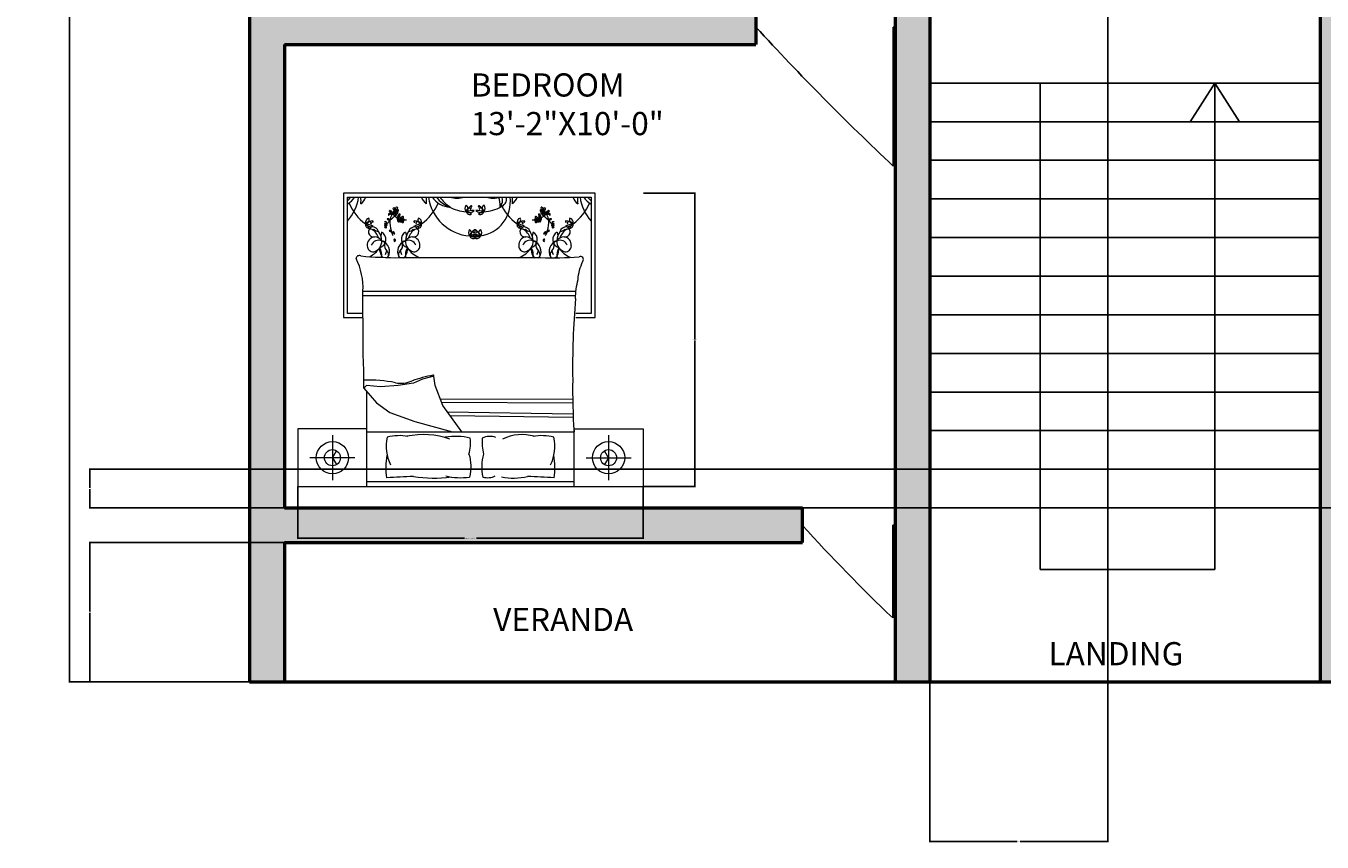
# Model space of a CAD drawing. Units: inches. Extents: x -17 to 536, y -817 to 53.
# Tile 1 of 9: x -17 to 319, y -817 to -606. Entities that reach past the tile are written whole.
import ezdxf

# ---------------------------------------------------------------- set-up
doc = ezdxf.new("R2010")
doc.units = ezdxf.units.IN
doc.header["$MEASUREMENT"] = 0
for name, color, linetype, lineweight in [('A-ANNO-DIMS', 2, 'Continuous', 18), ('A-AREA-IDEN', 7, 'Continuous', 18), ('A-DOOR', 4, 'Continuous', 25), ('A-FLOR-STRS', 7, 'Continuous', 25), ('A-FURN', 8, 'Continuous', 13), ('A-WALL', 7, 'Continuous', 50), ('A-WALL-PATT', 22, 'Continuous', 13)]:
    doc.layers.add(name, color=color, linetype=linetype, lineweight=lineweight)
doc.styles.get("Standard").update_dxf_attribs({"font": 'arial.ttf'})
doc.dimstyles.get("Standard").update_dxf_attribs({"dimtxt": 0.18, "dimasz": 0.18, "dimexe": 0.18, "dimexo": 0.0625, "dimgap": 0.09, "dimtad": 0, "dimtih": 1, "dimtoh": 1, "dimdec": 0, "dimzin": 0, "dimdsep": 46, "dimlunit": 3, "dimtxsty": 'Standard', "dimcen": 0.09, "dimadec": 0, "dimazin": 0, "dimtfac": 1, "dimtdec": 0, "dimtofl": 0, "dimtmove": 0, "dimatfit": 3, "dimfxl": 1, "dimtolj": 1, "dimtzin": 0, "dimarcsym": 0})

# ---------------------------------------------------------------- blocks, each defined once
blk = doc.blocks.new('*D2')
at = {"layer": 'A-ANNO-DIMS', "color": 0, "lineweight": -2, "transparency": 16777216}
for p, q in [((41.3, 11.55), (-5.38, 11.55)), ((-5.2, 11.37), (-5.2, -378.8)), ((-5.2, -775.27), (-5.2, -385.1)), ((41.3, -775.45), (-5.38, -775.45))]:
    blk.add_line(p, q, dxfattribs=at)
at = {"layer": 'A-ANNO-DIMS', "color": 0, "transparency": 16777216}
for points in [[(-5.23, 11.37), (-5.17, 11.37), (-5.2, 11.55)], [(-5.23, -775.27), (-5.17, -775.27), (-5.2, -775.45)]]:
    blk.add_solid(points, dxfattribs=at)
at = {"layer": 'Defpoints', "color": 0, "transparency": 16777216}
for p in [(41.37, 11.55), (-5.2, -775.45), (41.37, -775.45)]:
    blk.add_point(p, dxfattribs=at)
at = {"layer": 'A-ANNO-DIMS', "color": 0, "transparency": 16777216, "insert": (-5.2, -381.95), "char_height": 6, "attachment_point": 5}
blk.add_mtext('\\A1;65\'-7"', dxfattribs=at)
blk = doc.blocks.new('BED-WITH-NIGHTSTANDS-STANDARD')
for p, q in [((11.79, 75.95), (11.79, 43.78)), ((76.89, 75.95), (11.79, 75.95)), ((12.82, 74.91), (75.86, 74.91)), ((12.82, 44.81), (12.82, 74.91)), ((75.86, 74.91), (75.86, 44.81)), ((76.89, 43.78), (76.89, 75.95)), ((21.62, 65.86), (21.42, 64.85)), ((27.86, 65.86), (28.06, 64.85)), ((60.82, 65.86), (60.62, 64.85)), ((67.06, 65.86), (67.25, 64.85)), ((62.78, 59.23), (26.52, 59.23)), ((71.93, 50.46), (16.83, 50.46)), ((71.85, 49.35), (16.83, 49.35)), ((11.79, 43.78), (16.84, 43.78)), ((16.84, 44.81), (12.82, 44.81)), ((75.86, 44.81), (71.92, 44.81)), ((71.94, 43.78), (76.89, 43.78)), ((32.25, 27.79), (29.9, 26.71)), ((35.15, 28.52), (32.25, 27.79)), ((35.51, 26.17), (35.15, 28.52)), ((17.78, 26.17), (17.06, 25.44)), ((17.06, 25.44), (20.32, 21.65)), ((21.4, 25.8), (17.78, 26.17)), ((17.86, 0), (17.86, 24.51)), ((25.92, 26.17), (21.4, 25.8)), ((29.9, 26.71), (25.92, 26.17)), ((37.5, 20.92), (35.51, 26.17)), ((20.32, 21.65), (23.75, 19.12)), ((71.13, 22.47), (36.86, 22.61)), ((71.12, 21.55), (37.21, 21.69)), ((42.39, 14.11), (37.5, 20.92)), ((23.75, 19.12), (30.26, 16.77)), ((71.17, 18.74), (38.74, 19.2)), ((71.2, 17.82), (39.41, 18.27)), ((17.86, 14.11), (71.44, 14.11)), ((30.26, 16.77), (40, 14.11)), ((8.93, 13.28), (8.93, 1.61)), ((80.37, 13.28), (80.37, 1.61)), ((14.76, 7.44), (3.1, 7.44)), ((74.54, 7.44), (86.21, 7.44)), ((0, 0), (89.3, 0)), ((71.44, 1.15), (17.86, 1.15))]:
    blk.add_line(p, q)
for points in [[(16.87, 33.62, -0.001242), (16.83, 50.56, 0.127202), (15.04, 59.01)], [(71.82, 48.64, -0.056112), (72.47, 53.56, -0.095341), (73.73, 58.29)], [(22.99, 2.23, -0.074897), (23.1, 8.06, 0.472817)], [(44.23, 8.39, -0.14099), (44.41, 2.43, -0.235245)], [(48.05, 8.39, 0.14099), (47.87, 2.43, 0.235245)], [(66.31, 2.23, 0.074897), (66.2, 8.06, -0.472817)]]:
    blk.add_lwpolyline(points, format="xyb")
for points in [[(17.86, 14.88), (0, 14.88), (0, 0)], [(71.44, 0), (71.44, 14.88), (89.3, 14.88), (89.3, 0)], [(8.93, 7.44), (9.97, 9.25)], [(8.93, 7.44), (9.97, 5.64)], [(80.37, 7.44), (79.33, 9.25)], [(80.37, 7.44), (79.33, 5.64)]]:
    blk.add_lwpolyline(points)
for centre, radius in [((25.29, 71.49), 0.227), ((63.39, 71.49), 0.227), ((26.78, 69.09), 0.227), ((61.9, 69.09), 0.227), ((8.93, 7.44), 4.17), ((80.37, 7.44), 4.17), ((8.93, 7.44), 2.08), ((80.37, 7.44), 2.08)]:
    blk.add_circle(centre, radius)
for centre, radius, start, end in [((7.95, 79.1), 7.08, 313.5186, 323.6964), ((9.99, 78.04), 5.68, 299.8884, 326.5383), ((4.14, 76.48), 11.66, 318.1144, 352.255), ((13.17, 76.73), 4.74, 311.0454, 337.4453), ((0.19, 74.18), 16.13, 356.3481, 2.5919), ((36.31, 76.73), 4.74, 202.5547, 228.9546), ((49.3, 74.18), 16.13, 177.4081, 183.6519), ((45.35, 76.48), 11.66, 187.745, 265.5377), ((39.5, 78.04), 5.68, 213.4617, 268.728), ((41.54, 79.1), 7.08, 216.3036, 252.1496), ((45.26, 81.09), 10.53, 215.947, 235.9877), ((41.19, 81.04), 6.41, 252.9798, 286.4569), ((43.73, 84.35), 9.48, 264.3643, 265.6213), ((48.73, 90.84), 16.94, 250.0972, 250.2783), ((45.93, 73.79), 9.03, 278.1803, 7.1364), ((50.46, 81.04), 6.41, 253.5431, 287.0202), ((47.92, 84.35), 9.48, 274.3787, 275.6357), ((42.93, 90.84), 16.94, 289.7217, 289.9028), ((47.1, 72.96), 5.22, 353.3805, 21.883), ((51.89, 74.42), 2.09, 280.9261, 13.6102), ((50.32, 74.13), 2.65, 318.0951, 17.1391), ((39.38, 74.18), 16.13, 356.3481, 2.5919), ((52.37, 76.73), 4.74, 311.0454, 337.4453), ((75.51, 76.73), 4.74, 202.5547, 228.9546), ((88.49, 74.18), 16.13, 177.4081, 183.6519), ((84.54, 76.48), 11.66, 187.745, 221.8856), ((78.69, 78.04), 5.68, 213.4617, 240.1116), ((80.73, 79.1), 7.08, 216.3036, 226.4814), ((24.09, 77.63), 11.66, 201.4092, 235.6135), ((23.64, 70.33), 0.254, 123.0979, 213.1364), ((24.07, 69.96), 0.687, 92.3172, 160.5201), ((27.22, 64.73), 6.64, 121.1156, 124.8118), ((24, 70.22), 0.592, 82.6008, 147.1845), ((23.83, 71.16), 0.254, 55.6077, 145.6462), ((23.65, 70.61), 0.687, 21.7087, 93.0299), ((20.03, 65.71), 6.64, 53.6254, 57.3216), ((23.92, 70.2), 0.263, 45.7354, 121.1156), ((23.86, 70.79), 0.592, 342.8042, 79.6943), ((23.81, 70.85), 0.263, 338.2452, 53.6254), ((24.24, 70.68), 0.198, 158.2452, 340.6395), ((24.24, 70.53), 0.198, 225.7354, 48.1297), ((27.97, 72.33), 3.96, 201.7087, 206.2181), ((24.82, 69.63), 1.04, 40.9365, 112.7695), ((24.48, 69.98), 0.61, 49.3812, 95.5456), ((27.5, 68.52), 3.71, 137.5083, 145.9967), ((24.92, 70.22), 0.63, 61.1838, 141.6792), ((27.89, 73.45), 4.45, 220.182, 239.456), ((24.82, 71.92), 0.225, 134.3732, 211.9501), ((25.23, 72.18), 0.717, 211.9501, 255.2442), ((24.83, 71.66), 0.449, 8.5614, 112.5914), ((25.04, 71.17), 0.31, 88.5719, 233.8954), ((25.01, 71.09), 0.223, 228.2946, 6.2474), ((25.35, 71), 0.733, 229.3812, 289.9959), ((24.96, 71.68), 0.151, 352.868, 97.094), ((24.8, 71.35), 0.313, 298.8493, 359.9355), ((24.87, 71.09), 0.358, 4.2123, 48.1587), ((25.6, 71.91), 0.375, 100.9597, 208.7804), ((25.61, 71.14), 0.379, 183.635, 258.4363), ((24.88, 70.1), 0.753, 15.6484, 62.2957), ((25.56, 71.27), 0.217, 178.1325, 268.8919), ((26.01, 71.41), 0.69, 132.3896, 156.5724), ((25.71, 71.32), 0.372, 42.3208, 130.2111), ((25.79, 71.71), 0.47, 226.3462, 279.6513), ((25.29, 72.11), 0.529, 291.6382, 4.947), ((25.3, 70.84), 0.547, 7.4968, 71.2737), ((25.7, 72.2), 0.745, 254.2829, 276.9148), ((25.64, 72.14), 0.174, 4.947, 127.5263), ((25.68, 70.87), 0.176, 215.0752, 14.7644), ((25.31, 70.6), 1.04, 287.889, 359.722), ((25.84, 71.44), 0.196, 279.6513, 42.3208), ((26.61, 69.9), 0.733, 110.6625, 171.2773), ((25.66, 70.27), 0.753, 338.3627, 25.0101), ((25.39, 77.63), 11.66, 304.3865, 338.5908), ((44.45, 82.73), 11.66, 242.5854, 265.5377), ((44.5, 71.97), 1.29, 140.8855, 222.2127), ((43.03, 71.93), 0.974, 301.6373, 61.4609), ((44.5, 71.14), 0.954, 76.148, 182.2415), ((46.34, 70.15), 2.95, 121.989, 161.0841), ((45.99, 63.32), 8.16, 92.7418, 107.407), ((44.3, 72.78), 1.84, 245.6899, 314.4589), ((43.49, 69.11), 1.99, 44.6273, 88.5415), ((44.47, 71.37), 0.967, 196.1963, 296.9726), ((44.7, 71.94), 0.126, 140.0755, 76.148), ((44.85, 72.52), 0.145, 288.4408, 121.989), ((44.87, 72.45), 0.0704, 171.9833, 288.4408), ((45.67, 63.32), 8.16, 72.593, 87.2582), ((47.35, 72.78), 1.84, 225.5411, 294.3101), ((46.81, 72.52), 0.145, 58.011, 251.5592), ((48.16, 69.11), 1.99, 91.4585, 135.3727), ((47.18, 71.37), 0.967, 243.0274, 343.8037), ((46.78, 72.45), 0.0704, 251.5592, 8.0167), ((46.95, 71.89), 0.076, 103.9791, 39.8091), ((45.32, 70.15), 2.95, 18.9159, 58.011), ((47.16, 71.14), 0.954, 357.7585, 103.852), ((48.62, 71.93), 0.974, 118.5391, 238.3627), ((47.15, 71.97), 1.29, 317.7873, 39.1145), ((47.2, 82.73), 11.66, 274.4623, 297.4146), ((63.28, 77.63), 11.66, 201.4092, 235.6135), ((63.02, 70.27), 0.753, 154.9899, 201.6373), ((63.37, 70.6), 1.04, 180.278, 252.111), ((62.07, 69.9), 0.733, 8.7227, 69.3375), ((62.84, 71.44), 0.196, 137.6792, 260.3487), ((62.97, 71.32), 0.372, 49.7889, 137.6792), ((62.89, 71.71), 0.47, 260.3487, 313.6538), ((63.38, 70.84), 0.547, 108.7263, 172.5032), ((63, 70.87), 0.176, 165.2356, 324.9248), ((63.39, 72.11), 0.529, 175.053, 248.3618), ((63.04, 72.14), 0.174, 52.4737, 175.053), ((62.98, 72.2), 0.745, 263.0852, 285.7171), ((60.79, 73.45), 4.45, 300.544, 319.818), ((63.8, 70.1), 0.753, 117.7043, 164.3516), ((63.86, 69.63), 1.04, 67.2305, 139.0635), ((63.33, 71), 0.733, 250.0041, 310.6188), ((63.12, 71.27), 0.217, 271.1081, 1.8675), ((62.67, 71.41), 0.69, 23.4276, 47.6104), ((63.08, 71.91), 0.375, 331.2196, 79.0403), ((63.07, 71.14), 0.379, 281.5637, 356.365), ((63.85, 71.66), 0.449, 67.4086, 171.4386), ((63.81, 71.09), 0.358, 131.8413, 175.7877), ((63.67, 71.09), 0.223, 173.7526, 311.7054), ((63.75, 70.22), 0.63, 38.3208, 118.8162), ((63.72, 71.68), 0.151, 82.906, 187.132), ((63.88, 71.35), 0.313, 180.0645, 241.1507), ((63.45, 72.18), 0.717, 284.7558, 328.0499), ((63.64, 71.17), 0.31, 306.1046, 91.4281), ((64.2, 69.98), 0.61, 84.4544, 130.6188), ((61.17, 68.52), 3.71, 34.0033, 42.4917), ((63.86, 71.92), 0.225, 328.0499, 45.6268), ((64.81, 70.79), 0.592, 100.3057, 197.1958), ((64.44, 70.53), 0.198, 131.8703, 314.2646), ((64.44, 70.68), 0.198, 199.3605, 21.7548), ((60.71, 72.33), 3.96, 333.7819, 338.2913), ((65.03, 70.61), 0.687, 86.9701, 158.2913), ((64.76, 70.2), 0.263, 58.8844, 134.2646), ((64.86, 70.85), 0.263, 126.3746, 201.7548), ((64.68, 70.22), 0.592, 32.8155, 97.3992), ((64.6, 69.96), 0.687, 19.4799, 87.6828), ((64.85, 71.16), 0.254, 34.3538, 124.3923), ((68.65, 65.71), 6.64, 122.6784, 126.3746), ((61.46, 64.73), 6.64, 55.1882, 58.8844), ((65.04, 70.33), 0.254, 326.8636, 56.9021), ((64.59, 77.63), 11.66, 304.3865, 338.5908), ((18.77, 68.29), 1.29, 110.9613, 192.2885), ((18.44, 67.78), 0.967, 166.272, 267.0484), ((17.48, 68.98), 0.974, 271.7131, 31.5367), ((19.45, 65.79), 2.95, 92.0648, 131.1598), ((18.35, 67.57), 0.954, 46.2238, 152.3173), ((15.74, 60.05), 8.16, 62.8176, 77.4827), ((19, 69.09), 1.84, 215.7657, 284.5347), ((16.47, 66.31), 1.99, 14.7031, 58.6173), ((19.58, 65.93), 1.34, 109.1312, 279.736), ((18.92, 68.17), 0.126, 110.2817, 46.2238), ((19.26, 65.53), 1.67, 15.6955, 94.031), ((19.33, 68.52), 0.0704, 142.0591, 258.5166), ((19.35, 68.59), 0.145, 258.5166, 92.0648), ((22.68, 68.16), 0.375, 100.9597, 142.2379), ((22.37, 67.74), 0.227, 273.2768, 86.7232), ((22.69, 67.39), 0.379, 217.3642, 258.4363), ((22.64, 67.53), 0.217, 178.1325, 268.8919), ((23.09, 67.66), 0.69, 132.3896, 156.5724), ((22.78, 67.57), 0.372, 42.3208, 130.2111), ((22.87, 67.96), 0.47, 226.3462, 279.6513), ((22.36, 68.36), 0.529, 291.6382, 4.947), ((22.38, 67.09), 0.547, 7.4968, 71.2737), ((22.78, 68.45), 0.745, 254.2829, 276.9148), ((22.72, 68.39), 0.174, 4.947, 127.5263), ((22.75, 67.12), 0.176, 215.0752, 14.7644), ((17.62, 74.63), 8.48, 307.9541, 316.8459), ((22.91, 67.69), 0.196, 279.6513, 42.3208), ((23.13, 66.79), 2.52, 82.8698, 91.6736), ((23.48, 69.5), 0.469, 205.5379, 258.6744), ((22.81, 67.91), 1.41, 59.344, 79.7412), ((22.5, 67.92), 1.43, 43.6929, 51.7899), ((23.38, 68.86), 0.429, 355.7131, 81.6568), ((23.14, 68.48), 0.748, 27.3659, 59.344), ((23.71, 68.98), 0.182, 202.5583, 304.2343), ((31.19, 68.33), 7.4, 176.1723, 196.4158), ((27.5, 68.52), 3.71, 150.7959, 175.244), ((32.84, 60.63), 12.2, 127.8256, 137.7588), ((25.28, 70.11), 0.61, 305.1128, 351.2773), ((25.59, 68.99), 0.63, 3.8774, 87.1501), ((25.15, 69.23), 0.61, 352.0748, 38.2393), ((25.04, 68.75), 1.04, 343.6301, 55.4631), ((26.48, 69.05), 0.733, 172.0748, 232.6895), ((25.77, 70.21), 0.63, 271.4625, 339.4747), ((25.47, 68.96), 0.753, 318.342, 4.9894), ((26.3, 69.52), 0.225, 134.3732, 211.9501), ((27.89, 73.45), 4.45, 246.1523, 246.9499), ((26.72, 69.78), 0.717, 211.9501, 255.2442), ((26.32, 69.27), 0.449, 8.5614, 112.5914), ((26.53, 68.78), 0.31, 88.5719, 233.8954), ((26.5, 68.69), 0.223, 228.2946, 6.2474), ((26.44, 69.28), 0.151, 352.868, 97.094), ((26.29, 68.96), 0.313, 298.8493, 359.9355), ((26.36, 68.69), 0.358, 4.2123, 48.1587), ((27.09, 69.51), 0.375, 100.9597, 208.7804), ((27.1, 68.74), 0.379, 183.635, 258.4363), ((27.05, 68.88), 0.217, 178.1325, 268.8919), ((27.5, 69.01), 0.69, 132.3896, 156.5724), ((27.19, 68.93), 0.372, 42.3208, 130.2111), ((27.28, 69.31), 0.47, 226.3462, 279.6513), ((26.77, 69.71), 0.529, 291.6382, 4.947), ((26.79, 68.44), 0.547, 7.4968, 71.2737), ((27.19, 69.8), 0.745, 254.2829, 276.9148), ((27.13, 69.74), 0.174, 4.947, 127.5263), ((27.16, 68.47), 0.176, 215.0752, 14.7644), ((27.32, 69.04), 0.196, 279.6513, 42.3208), ((27.89, 73.45), 4.45, 265.2415, 272.8929), ((30.23, 65.53), 1.67, 85.969, 164.3045), ((29.91, 65.93), 1.34, 260.264, 70.8688), ((30.14, 68.59), 0.145, 87.9352, 281.4834), ((30.48, 69.09), 1.84, 255.4653, 324.2343), ((33.75, 60.05), 8.16, 102.5173, 117.1824), ((30.04, 65.79), 2.95, 48.8402, 87.9352), ((30.16, 68.52), 0.0704, 281.4834, 37.9409), ((31.14, 67.57), 0.954, 27.6827, 133.7762), ((30.58, 68.12), 0.076, 133.7729, 69.7333), ((32.01, 68.98), 0.974, 148.4633, 268.2869), ((31.04, 67.78), 0.967, 272.9516, 13.728), ((33.02, 66.31), 1.99, 121.3827, 165.2969), ((30.72, 68.29), 1.29, 347.7115, 69.0387), ((57.96, 68.29), 1.29, 110.9613, 192.2885), ((57.64, 67.78), 0.967, 166.272, 267.0484), ((56.67, 68.98), 0.974, 271.7131, 31.5367), ((58.64, 65.79), 2.95, 92.0648, 131.1598), ((57.54, 67.57), 0.954, 46.2238, 152.3173), ((55.66, 66.31), 1.99, 14.7031, 58.6173), ((58.19, 69.09), 1.84, 215.7657, 284.5347), ((54.93, 60.05), 8.16, 62.8176, 77.4827), ((58.77, 65.93), 1.34, 109.1312, 279.736), ((58.12, 68.17), 0.126, 110.2817, 46.2238), ((58.45, 65.53), 1.67, 15.6955, 94.031), ((58.52, 68.52), 0.0704, 142.0591, 258.5166), ((58.54, 68.59), 0.145, 258.5166, 92.0648), ((60.79, 73.45), 4.45, 267.1071, 274.7585), ((61.36, 69.04), 0.196, 137.6792, 260.3487), ((61.49, 68.93), 0.372, 49.7889, 137.6792), ((61.4, 69.31), 0.47, 260.3487, 313.6538), ((61.52, 68.47), 0.176, 165.2356, 324.9248), ((61.89, 68.44), 0.547, 108.7263, 172.5032), ((61.55, 69.74), 0.174, 52.4737, 175.053), ((61.91, 69.71), 0.529, 175.053, 248.3618), ((61.49, 69.8), 0.745, 263.0852, 285.7171), ((61.63, 68.88), 0.217, 271.1081, 1.8675), ((61.18, 69.01), 0.69, 23.4276, 47.6104), ((61.59, 69.51), 0.375, 331.2196, 79.0403), ((61.58, 68.74), 0.379, 281.5637, 356.365), ((62.36, 69.27), 0.449, 67.4086, 171.4386), ((62.32, 68.69), 0.358, 131.8413, 175.7877), ((62.18, 68.69), 0.223, 173.7526, 311.7054), ((62.23, 69.28), 0.151, 82.906, 187.132), ((62.39, 68.96), 0.313, 180.0645, 241.1507), ((61.96, 69.78), 0.717, 284.7558, 328.0499), ((62.15, 68.78), 0.31, 306.1046, 91.4281), ((62.91, 70.21), 0.63, 200.5253, 268.5375), ((63.21, 68.96), 0.753, 175.0106, 221.658), ((63.08, 68.99), 0.63, 92.8499, 176.1226), ((62.38, 69.52), 0.225, 328.0499, 45.6268), ((60.79, 73.45), 4.45, 293.0501, 293.8477), ((63.64, 68.75), 1.04, 124.5369, 196.3699), ((62.2, 69.05), 0.733, 307.3105, 7.9252), ((63.4, 70.11), 0.61, 188.7227, 234.8872), ((63.53, 69.23), 0.61, 141.7607, 187.9252), ((55.84, 60.63), 12.2, 42.2412, 52.1744), ((61.17, 68.52), 3.71, 4.756, 29.2041), ((57.49, 68.33), 7.4, 343.5842, 3.8277), ((65.3, 68.86), 0.429, 98.3432, 184.2869), ((65.53, 68.48), 0.748, 120.656, 152.6341), ((64.97, 68.98), 0.182, 235.7657, 337.4417), ((71.06, 74.63), 8.48, 223.1541, 232.0459), ((66.18, 67.92), 1.43, 128.2101, 136.3071), ((65.87, 67.91), 1.41, 100.2588, 120.656), ((65.55, 66.79), 2.52, 88.3264, 97.1302), ((65.2, 69.5), 0.469, 281.3256, 334.4621), ((65.76, 67.69), 0.196, 137.6792, 260.3487), ((65.89, 67.57), 0.372, 49.7889, 137.6792), ((65.81, 67.96), 0.47, 260.3487, 313.6538), ((66.3, 67.09), 0.547, 108.7263, 172.5032), ((65.92, 67.12), 0.176, 165.2356, 324.9248), ((65.96, 68.39), 0.174, 52.4737, 175.053), ((66.31, 68.36), 0.529, 175.053, 248.3618), ((65.9, 68.45), 0.745, 263.0852, 285.7171), ((66.04, 67.53), 0.217, 271.1081, 1.8675), ((65.59, 67.66), 0.69, 23.4276, 47.6104), ((66, 68.16), 0.375, 37.7621, 79.0403), ((65.99, 67.39), 0.379, 281.5637, 322.6358), ((66.31, 67.74), 0.227, 93.2768, 266.7232), ((69.42, 65.53), 1.67, 85.969, 164.3045), ((69.1, 65.93), 1.34, 260.264, 70.8688), ((69.33, 68.59), 0.145, 87.9352, 281.4834), ((72.94, 60.05), 8.16, 102.5173, 117.1824), ((69.68, 69.09), 1.84, 255.4653, 324.2343), ((69.23, 65.79), 2.95, 48.8402, 87.9352), ((69.35, 68.52), 0.0704, 281.4834, 37.9409), ((70.33, 67.57), 0.954, 27.6827, 133.7762), ((69.77, 68.12), 0.076, 133.7729, 69.7333), ((71.2, 68.98), 0.974, 148.4633, 268.2869), ((72.21, 66.31), 1.99, 121.3827, 165.2969), ((70.23, 67.78), 0.967, 272.9516, 13.728), ((69.91, 68.29), 1.29, 347.7115, 69.0387), ((20.07, 62.49), 2.13, 97.1143, 185.0551), ((19.3, 67.38), 0.821, 216.7319, 296.0245), ((20.91, 61.68), 2.07, 68.5779, 158.4181), ((16.92, 62.98), 4.22, 18.2955, 58.7386), ((21.06, 67.75), 1.78, 218.4175, 263.8338), ((19.7, 62.02), 2.59, 35.9599, 87.6409), ((16.88, 63.32), 4.79, 3.4924, 33.7117), ((20.52, 63.93), 2.22, 286.8663, 60.0915), ((23.66, 63.78), 2.52, 82.8698, 91.6736), ((24.01, 66.5), 0.469, 205.5379, 258.6744), ((23.34, 64.91), 1.41, 59.344, 79.7412), ((23.03, 64.91), 1.43, 43.6929, 51.7899), ((23.91, 65.86), 0.429, 355.7131, 81.6568), ((23.68, 65.48), 0.748, 27.3659, 59.344), ((24.24, 65.97), 0.182, 202.5583, 304.2343), ((31.19, 68.33), 7.4, 200.1059, 206.9968), ((24.57, 65.46), 0.429, 36.5232, 122.4668), ((24.35, 65.08), 0.748, 58.836, 90.8141), ((24.52, 65.8), 0.182, 173.9457, 275.6216), ((24.16, 64.24), 1.43, 66.3901, 74.4871), ((25.09, 65.85), 0.469, 219.5056, 272.6421), ((24.01, 64.51), 1.41, 38.4388, 58.836), ((25, 63.84), 0.172, 79.5616, 257.2949), ((22.86, 64.26), 2.52, 26.5064, 35.3102), ((24.98, 63.73), 0.28, 259.5864, 79.5616), ((28.97, 63.93), 2.22, 119.9085, 253.1337), ((29.79, 62.02), 2.59, 92.3591, 144.0401), ((32.6, 63.32), 4.79, 146.2883, 176.5076), ((28.58, 61.68), 2.07, 21.5819, 111.4221), ((32.56, 62.98), 4.22, 121.2614, 161.7045), ((28.42, 67.75), 1.78, 276.1662, 321.5825), ((29.42, 62.49), 2.13, 354.9449, 82.8857), ((30.18, 67.38), 0.821, 243.9755, 323.2681), ((45.4, 65.72), 1.29, 140.8855, 222.2127), ((43.93, 65.68), 0.974, 301.6373, 61.4609), ((47.23, 63.9), 2.95, 121.989, 161.0841), ((45.39, 64.89), 0.954, 76.148, 182.2415), ((45.2, 66.54), 1.84, 245.6899, 314.4589), ((46.88, 57.07), 8.16, 92.7418, 107.407), ((45.37, 65.13), 0.967, 196.1963, 296.9726), ((44.39, 62.86), 1.99, 44.6273, 88.5415), ((46.46, 66.54), 1.84, 225.5411, 294.3101), ((44.78, 57.07), 8.16, 72.593, 87.2582), ((45.59, 65.7), 0.126, 140.0755, 76.148), ((45.74, 66.28), 0.145, 288.4408, 121.989), ((45.77, 66.21), 0.0704, 171.9833, 288.4408), ((45.91, 66.28), 0.145, 58.011, 251.5592), ((46.29, 65.13), 0.967, 243.0274, 343.8037), ((47.27, 62.86), 1.99, 91.4585, 135.3727), ((45.89, 66.21), 0.0704, 251.5592, 8.0167), ((46.05, 65.65), 0.076, 103.9791, 39.8091), ((44.43, 63.9), 2.95, 18.9159, 58.011), ((46.26, 64.89), 0.954, 357.7585, 103.852), ((47.73, 65.68), 0.974, 118.5391, 238.3627), ((46.26, 65.72), 1.29, 317.7873, 39.1145), ((59.26, 62.49), 2.13, 97.1143, 185.0551), ((58.5, 67.38), 0.821, 216.7319, 296.0245), ((60.1, 61.68), 2.07, 68.5779, 158.4181), ((56.12, 62.98), 4.22, 18.2955, 58.7386), ((60.25, 67.75), 1.78, 218.4175, 263.8338), ((58.89, 62.02), 2.59, 35.9599, 87.6409), ((56.08, 63.32), 4.79, 3.4924, 33.7117), ((59.71, 63.93), 2.22, 286.8663, 60.0915), ((63.7, 63.73), 0.28, 100.4384, 280.4136), ((64.67, 64.51), 1.41, 121.164, 141.5612), ((65.82, 64.26), 2.52, 144.6898, 153.4936), ((63.59, 65.85), 0.469, 267.3579, 320.4944), ((63.68, 63.84), 0.172, 282.7051, 100.4384), ((64.11, 65.46), 0.429, 57.5332, 143.4768), ((64.33, 65.08), 0.748, 89.1859, 121.164), ((64.52, 64.24), 1.43, 105.5129, 113.6099), ((57.49, 68.33), 7.4, 333.0032, 339.8941), ((64.16, 65.8), 0.182, 264.3784, 6.0543), ((64.77, 65.86), 0.429, 98.3432, 184.2869), ((65, 65.48), 0.748, 120.656, 152.6341), ((64.44, 65.97), 0.182, 235.7657, 337.4417), ((65.65, 64.91), 1.43, 128.2101, 136.3071), ((65.34, 64.91), 1.41, 100.2588, 120.656), ((65.02, 63.78), 2.52, 88.3264, 97.1302), ((64.67, 66.5), 0.469, 281.3256, 334.4621), ((68.16, 63.93), 2.22, 119.9085, 253.1337), ((68.98, 62.02), 2.59, 92.3591, 144.0401), ((71.8, 63.32), 4.79, 146.2883, 176.5076), ((67.77, 61.68), 2.07, 21.5819, 111.4221), ((71.76, 62.98), 4.22, 121.2614, 161.7045), ((67.62, 67.75), 1.78, 276.1662, 321.5825), ((68.61, 62.49), 2.13, 354.9449, 82.8857), ((69.38, 67.38), 0.821, 243.9755, 323.2681), ((19.45, 62.27), 1.51, 178.9462, 275.5144), ((15.52, 65.52), 6.76, 296.7003, 326.3329), ((18.99, 63.39), 2.69, 283.079, 4.7067), ((24.57, 61.5), 3.44, 175.2696, 214.215), ((17.99, 59.89), 3.7, 350.8446, 31.1782), ((24.57, 61.5), 3.44, 143.6555, 147.2989), ((21.92, 63), 0.554, 344.8529, 102.6959), ((20.86, 60.85), 2.85, 330.8249, 70.7178), ((24.22, 62.38), 1.83, 164.8529, 228.4347), ((20.43, 61.37), 2.57, 330.0851, 352.564), ((22.12, 60.01), 1.34, 336.1646, 48.4347), ((28.63, 60.85), 2.85, 109.2822, 209.1751), ((27.36, 60.01), 1.34, 131.5653, 203.8354), ((25.26, 62.38), 1.83, 311.5653, 15.1471), ((29.06, 61.37), 2.57, 187.436, 209.9149), ((27.56, 63), 0.554, 77.3041, 195.1471), ((24.91, 61.5), 3.44, 32.7011, 36.3445), ((24.91, 61.5), 3.44, 325.785, 4.7304), ((31.49, 59.89), 3.7, 148.8218, 190.2867), ((30.5, 63.39), 2.69, 175.2933, 256.921), ((33.97, 65.52), 6.76, 213.6671, 248.5059), ((30.03, 62.27), 1.51, 264.4856, 1.0538), ((58.65, 62.27), 1.51, 178.9462, 275.5144), ((54.71, 65.52), 6.76, 291.4941, 326.3329), ((58.18, 63.39), 2.69, 283.079, 4.7067), ((63.77, 61.5), 3.44, 175.2696, 214.215), ((57.19, 59.89), 3.7, 349.7133, 31.1782), ((63.77, 61.5), 3.44, 143.6555, 147.2989), ((61.11, 63), 0.554, 344.8529, 102.6959), ((60.05, 60.85), 2.85, 330.8249, 70.7178), ((63.42, 62.38), 1.83, 164.8529, 228.4347), ((59.62, 61.37), 2.57, 330.0851, 352.564), ((61.32, 60.01), 1.34, 336.1646, 48.4347), ((67.82, 60.85), 2.85, 109.2822, 209.1751), ((66.56, 60.01), 1.34, 131.5653, 203.8354), ((64.46, 62.38), 1.83, 311.5653, 15.1471), ((68.25, 61.37), 2.57, 187.436, 209.9149), ((66.76, 63), 0.554, 77.3041, 195.1471), ((64.11, 61.5), 3.44, 32.7011, 36.3445), ((64.11, 61.5), 3.44, 325.785, 4.7304), ((70.68, 59.89), 3.7, 148.8218, 190.751), ((69.69, 63.39), 2.69, 175.2933, 256.921), ((73.16, 65.52), 6.76, 213.6671, 246.3547), ((69.23, 62.27), 1.51, 264.4856, 1.0538), ((15.86, 58.95), 0.824, 62.6588, 176.02), ((25.46, 152.19), 92.96, 264.3113, 270.6567), ((22.58, 60.22), 1.08, 217.675, 239.9707), ((22.58, 60.22), 1.08, 296.442, 315.5483), ((26.91, 60.22), 1.08, 224.4517, 246.771), ((26.91, 60.22), 1.08, 293.2856, 322.325), ((61.77, 60.22), 1.08, 217.675, 246.7144), ((61.77, 60.22), 1.08, 293.2856, 315.5483), ((65.51, 146.09), 86.9, 268.1965, 274.7598), ((66.1, 60.22), 1.08, 224.4517, 253.3657), ((66.1, 60.22), 1.08, 287.4186, 322.325), ((73.05, 58.74), 0.814, 326.1736, 113.4781), ((280.38, 30.86), 209.31, 175.1265, 180.8855), ((-64.82, 27.66), 81.91, 358.447, 4.1706), ((18.59, -6.18), 33.7, 78.6608, 92.5481), ((26.65, 33.99), 7.27, 258.6608, 293.7384), ((41.35, -5.23), 34.63, 100.6617, 109.8806), ((34.95, 28.59), 0.215, 340.2464, 91.1377), ((231.53, 25.03), 160.46, 179.0718, 183.9), ((32.48, -7.33), 20.76, 70.7385, 101.9603), ((57.96, 2.06), 11.37, 73.8254, 116.1239), ((34.37, 10.4), 11.51, 168.2417, 204.8684), ((26.18, 1.18), 11.97, 78.9631, 104.8961), ((40.88, -2.79), 15.75, 76.3762, 100.1383), ((33.71, 11.37), 10.94, 344.1707, 5.9871), ((58.57, 11.37), 10.94, 174.0129, 195.8293), ((49.69, 8.22), 4.73, 71.4593, 114.9817), ((63.13, 1.18), 11.97, 75.1039, 101.0369), ((54.94, 10.4), 11.51, 335.1316, 11.7583), ((72.21, -847.63), 851.28, 92.85022, 93.31479), ((35.23, 34.54), 32.39, 260.503, 277.7804), ((42.07, 18.17), 15.91, 256.04, 278.4751), ((49.09, 6.68), 4.42, 253.8974, 296.6563), ((55.71, 17.85), 15.7, 258.8159, 283.6573), ((17.09, -847.63), 851.28, 86.68521, 87.14978)]:
    blk.add_arc(centre, radius, start, end)
blk = doc.blocks.new('*D18')
at = {"layer": 'A-ANNO-DIMS', "color": 0, "lineweight": -2, "transparency": 16777216}
for p, q in [((53.86, -724.95), (53.86, -738.47)), ((143.16, -724.95), (143.16, -738.47)), ((54.04, -738.29), (96.98, -738.29)), ((142.98, -738.29), (100.05, -738.29))]:
    blk.add_line(p, q, dxfattribs=at)
at = {"layer": 'A-ANNO-DIMS', "color": 0, "transparency": 16777216}
for points in [[(54.04, -738.26), (54.04, -738.32), (53.86, -738.29)], [(142.98, -738.26), (142.98, -738.32), (143.16, -738.29)]]:
    blk.add_solid(points, dxfattribs=at)
at = {"layer": 'Defpoints', "color": 0, "transparency": 16777216}
for p in [(53.86, -724.89), (143.16, -724.89), (143.16, -738.29)]:
    blk.add_point(p, dxfattribs=at)
at = {"layer": 'A-ANNO-DIMS', "color": 0, "transparency": 16777216, "insert": (98.51, -738.29), "char_height": 0.18, "attachment_point": 5}
blk.add_mtext('\\A1;BED SET A 7\'-5 1/2" TYP.', dxfattribs=at)
blk = doc.blocks.new('*D19')
at = {"layer": 'A-ANNO-DIMS', "color": 0, "lineweight": -2, "transparency": 16777216}
for p, q in [((143.23, -648.95), (156.74, -648.95)), ((156.56, -649.13), (156.56, -686.74)), ((156.56, -724.71), (156.56, -687.1)), ((143.23, -724.89), (156.74, -724.89))]:
    blk.add_line(p, q, dxfattribs=at)
at = {"layer": 'A-ANNO-DIMS', "color": 0, "transparency": 16777216}
for points in [[(156.53, -649.13), (156.59, -649.13), (156.56, -648.95)], [(156.53, -724.71), (156.59, -724.71), (156.56, -724.89)]]:
    blk.add_solid(points, dxfattribs=at)
at = {"layer": 'Defpoints', "color": 0, "transparency": 16777216}
for p in [(143.16, -648.95), (156.56, -648.95), (143.16, -724.89)]:
    blk.add_point(p, dxfattribs=at)
at = {"layer": 'A-ANNO-DIMS', "color": 0, "transparency": 16777216, "insert": (156.56, -686.92), "char_height": 0.18, "attachment_point": 5}
blk.add_mtext('\\A1;6\'-4" TYP.', dxfattribs=at)
blk = doc.blocks.new('*D37')
at = {"layer": 'A-ANNO-DIMS', "color": 0, "lineweight": -2, "transparency": 16777216}
for p, q in [((50.3, -739.45), (-0.16, -739.45)), ((0.02, -739.63), (0.02, -757.27)), ((0.02, -775.27), (0.02, -757.63)), ((50.3, -775.45), (-0.16, -775.45))]:
    blk.add_line(p, q, dxfattribs=at)
at = {"layer": 'A-ANNO-DIMS', "color": 0, "transparency": 16777216}
for points in [[(-0.01, -739.63), (0.05, -739.63), (0.02, -739.45)], [(-0.01, -775.27), (0.05, -775.27), (0.02, -775.45)]]:
    blk.add_solid(points, dxfattribs=at)
at = {"layer": 'Defpoints', "color": 0, "transparency": 16777216}
for p in [(50.37, -739.45), (0.02, -775.45), (50.37, -775.45)]:
    blk.add_point(p, dxfattribs=at)
at = {"layer": 'A-ANNO-DIMS', "color": 0, "transparency": 16777216, "insert": (0.02, -757.45), "char_height": 0.18, "attachment_point": 5}
blk.add_mtext('\\A1;3\'-0"', dxfattribs=at)
blk = doc.blocks.new('*D38')
at = {"layer": 'A-ANNO-DIMS', "color": 0, "lineweight": -2, "transparency": 16777216}
for p, q in [((318.3, -720.45), (-0.16, -720.45)), ((0.02, -720.63), (0.02, -725.27)), ((0.02, -730.27), (0.02, -725.63)), ((318.3, -730.45), (-0.16, -730.45))]:
    blk.add_line(p, q, dxfattribs=at)
at = {"layer": 'A-ANNO-DIMS', "color": 0, "transparency": 16777216}
for points in [[(-0.01, -720.63), (0.05, -720.63), (0.02, -720.45)], [(-0.01, -730.27), (0.05, -730.27), (0.02, -730.45)]]:
    blk.add_solid(points, dxfattribs=at)
at = {"layer": 'Defpoints', "color": 0, "transparency": 16777216}
for p in [(0.02, -720.45), (318.37, -720.45), (318.37, -730.45)]:
    blk.add_point(p, dxfattribs=at)
at = {"layer": 'A-ANNO-DIMS', "color": 0, "transparency": 16777216, "insert": (0.02, -725.45), "char_height": 0.18, "attachment_point": 5}
blk.add_mtext('\\A1;0\'-10"', dxfattribs=at)
blk = doc.blocks.new('*D39')
at = {"layer": 'A-ANNO-DIMS', "color": 0, "lineweight": -2, "transparency": 16777216}
for p, q in [((217.43, -730.45), (535.9, -730.45)), ((535.72, -730.63), (535.72, -752.77)), ((535.72, -775.27), (535.72, -753.13)), ((217.43, -775.45), (535.9, -775.45))]:
    blk.add_line(p, q, dxfattribs=at)
at = {"layer": 'A-ANNO-DIMS', "color": 0, "transparency": 16777216}
for points in [[(535.69, -730.63), (535.75, -730.63), (535.72, -730.45)], [(535.69, -775.27), (535.75, -775.27), (535.72, -775.45)]]:
    blk.add_solid(points, dxfattribs=at)
at = {"layer": 'Defpoints', "color": 0, "transparency": 16777216}
for p in [(217.37, -730.45), (217.37, -775.45), (535.72, -775.45)]:
    blk.add_point(p, dxfattribs=at)
at = {"layer": 'A-ANNO-DIMS', "color": 0, "transparency": 16777216, "insert": (535.72, -752.95), "char_height": 0.18, "attachment_point": 5}
blk.add_mtext('\\A1;3\'-9"', dxfattribs=at)
blk = doc.blocks.new('*D40')
at = {"layer": 'A-ANNO-DIMS', "color": 0, "lineweight": -2, "transparency": 16777216}
for p, q in [((217.37, -544.51), (217.37, -816.98)), ((263.37, -553.51), (263.37, -816.98)), ((217.55, -816.8), (239.97, -816.8)), ((263.19, -816.8), (240.76, -816.8))]:
    blk.add_line(p, q, dxfattribs=at)
at = {"layer": 'A-ANNO-DIMS', "color": 0, "transparency": 16777216}
for points in [[(217.55, -816.77), (217.55, -816.83), (217.37, -816.8)], [(263.19, -816.77), (263.19, -816.83), (263.37, -816.8)]]:
    blk.add_solid(points, dxfattribs=at)
at = {"layer": 'Defpoints', "color": 0, "transparency": 16777216}
for p in [(217.37, -544.45), (263.37, -553.45), (263.37, -816.8)]:
    blk.add_point(p, dxfattribs=at)
at = {"layer": 'A-ANNO-DIMS', "color": 0, "transparency": 16777216, "insert": (240.37, -816.8), "char_height": 0.18, "attachment_point": 5}
blk.add_mtext('\\A1;3\'-10"', dxfattribs=at)

msp = doc.modelspace()

# ---------------------------------------------------------------- hatches: boundary and pattern name
at = {"layer": 'A-WALL-PATT'}
h = msp.add_hatch(color=256, dxfattribs=at)
h.dxf.hatch_style = 1
h.paths.add_polyline_path([(217.37, -544.45), (208.37, -544.45), (208.37, -775.45), (217.37, -775.45)], flags=17)
h.paths.add_polyline_path([(327.37, -544.45), (318.37, -544.45), (318.37, -775.45), (327.37, -775.45)], flags=17)
h.paths.add_polyline_path([(494.37, 11.55), (41.37, 11.55), (41.37, -775.45), (50.37, -775.45), (50.37, -739.45), (184.37, -739.45), (184.37, -730.45), (50.37, -730.45), (50.37, -610.45), (172.37, -610.45), (172.37, -601.45), (155.37, -601.45), (155.37, -577.45), (146.37, -577.45), (146.37, -601.45), (50.37, -601.45), (50.37, -553.45), (172.37, -553.45), (172.37, -544.45), (50.37, -544.45), (50.37, -436.45), (191.37, -436.45), (191.37, -319.45), (182.37, -319.45), (182.37, -427.45), (50.37, -427.45), (50.37, -283.45), (98.37, -283.45), (98.37, -274.45), (50.37, -274.45), (50.37, -219.45), (122.37, -219.45), (122.37, -283.45), (191.37, -283.45), (191.37, -274.45), (131.37, -274.45), (131.37, -219.45), (131.37, -150.45), (146.37, -150.45), (146.37, -141.45), (122.37, -141.45), (122.37, -210.45), (50.37, -210.45), (50.37, -150.45), (98.37, -150.45), (98.37, -141.45), (50.37, -141.45), (50.37, 2.55), (182.37, 2.55), (182.37, -150.45), (191.37, -150.45), (191.37, 2.55), (263.37, 2.55), (263.37, -141.45), (227.37, -141.45), (227.37, -150.45), (263.37, -150.45), (263.37, -553.45), (272.37, -553.45), (272.37, -150.45), (308.37, -150.45), (308.37, -141.45), (272.37, -141.45), (272.37, 2.55), (344.37, 2.55), (344.37, -150.45), (353.37, -150.45), (353.37, 2.55), (485.37, 2.55), (485.37, -141.45), (437.37, -141.45), (437.37, -150.45), (485.37, -150.45), (485.37, -210.45), (413.37, -210.45), (413.37, -141.45), (389.37, -141.45), (389.37, -150.45), (404.37, -150.45), (404.37, -219.45), (404.37, -274.45), (353.37, -274.45), (344.37, -274.45), (344.37, -283.45), (353.37, -283.45), (413.37, -283.45), (413.37, -219.45), (485.37, -219.45), (485.37, -274.45), (437.37, -274.45), (437.37, -283.45), (485.37, -283.45), (485.37, -427.45), (353.37, -427.45), (353.37, -319.45), (344.37, -319.45), (344.37, -436.45), (485.37, -436.45), (485.37, -544.45), (363.37, -544.45), (363.37, -553.45), (485.37, -553.45), (485.37, -601.45), (389.37, -601.45), (389.37, -577.45), (380.37, -577.45), (380.37, -601.45), (363.37, -601.45), (363.37, -610.45), (485.37, -610.45), (485.37, -730.45), (351.37, -730.45), (351.37, -739.45), (485.37, -739.45), (485.37, -775.45), (494.37, -775.45)])

# ---------------------------------------------------------------- linework, layer by layer
at = {"layer": 'A-DOOR'}
for p, q in [((207.89, -605.95), (208.37, -605.95)), ((207.89, -605.95), (207.89, -641.95)), ((207.76, -734.95), (208.37, -734.95)), ((207.76, -734.95), (207.76, -758.95))]:
    msp.add_line(p, q, dxfattribs=at)
for centre, radius, start, end in [((673.55, -146.92), 679.63, 222.48632, 226.75113), ((529.73, -421.69), 466.28, 222.2093, 226.3286)]:
    msp.add_arc(centre, radius, start, end, dxfattribs=at)
at = {"layer": 'A-FLOR-STRS'}
for p, q in [((217.37, -620.45), (318.37, -620.45)), ((245.93, -620.45), (245.93, -746.44)), ((291.08, -620.45), (284.74, -630.45)), ((291.08, -746.44), (291.08, -620.45)), ((291.08, -620.45), (297.43, -630.45)), ((217.37, -630.45), (318.37, -630.45)), ((217.37, -640.45), (318.37, -640.45)), ((217.37, -650.45), (318.37, -650.45)), ((217.37, -660.45), (318.37, -660.45)), ((217.37, -670.45), (318.37, -670.45)), ((217.37, -680.45), (318.37, -680.45)), ((217.37, -690.45), (318.37, -690.45)), ((217.37, -700.45), (318.37, -700.45)), ((217.37, -710.45), (318.37, -710.45)), ((217.37, -720.45), (318.37, -720.45)), ((217.37, -730.45), (318.37, -730.45)), ((245.93, -746.44), (291.08, -746.44))]:
    msp.add_line(p, q, dxfattribs=at)
at = {"layer": 'A-WALL'}
for p, q in [((41.37, 11.55), (41.37, -775.45)), ((208.37, -544.45), (208.37, -775.45)), ((217.37, -544.45), (217.37, -775.45)), ((318.37, -544.45), (318.37, -775.45)), ((172.37, -601.45), (172.37, -610.45)), ((50.37, -610.45), (172.37, -610.45)), ((50.37, -610.45), (50.37, -730.45)), ((50.37, -730.45), (184.37, -730.45)), ((184.37, -739.45), (184.37, -730.45)), ((50.37, -739.45), (184.37, -739.45)), ((50.37, -739.45), (50.37, -775.45)), ((41.37, -775.45), (353.37, -775.45))]:
    msp.add_line(p, q, dxfattribs=at)

# ---------------------------------------------------------------- block references
at = {"layer": 'A-FURN'}
msp.add_blockref('BED-WITH-NIGHTSTANDS-STANDARD', (53.86, -724.89), dxfattribs=at)

# ---------------------------------------------------------------- texts
at = {"layer": 'A-AREA-IDEN', "char_height": 6, "attachment_point": 1}
for s, insert in [('BEDROOM\\P13\'-2"X10\'-0"', (98.57, -617.94)), ('VERANDA', (104.37, -756.36)), ('LANDING', (248.04, -765.2))]:
    msp.add_mtext(s, dxfattribs=dict(at, insert=insert))

# ---------------------------------------------------------------- dimensions: what is measured, and where the dimension line sits
at = {"layer": 'A-ANNO-DIMS'}
for base, p1, p2, override, picture, middle in [((-5.2, -775.45), (41.37, 11.55), (41.37, -775.45), {"dimtxt": 6, "dimclrd": 0, "dimclre": 0, "dimclrt": 0}, '*D2', (-5.2, -381.95)), ((0.02, -720.45), (318.37, -730.45), (318.37, -720.45), {"dimdec": 1, "dimlfac": 1, "dimrnd": 0, "dimzin": 1, "dimdsep": 46, "dimlunit": 4, "dimfrac": 2}, '*D38', (0.02, -725.45)), ((535.72, -775.45), (217.37, -730.45), (217.37, -775.45), {"dimdec": 1, "dimlfac": 1, "dimrnd": 0, "dimzin": 1, "dimdsep": 46, "dimlunit": 4, "dimfrac": 2}, '*D39', (535.72, -752.95)), ((0.02, -775.45), (50.37, -739.45), (50.37, -775.45), {"dimdec": 1, "dimlfac": 1, "dimrnd": 0, "dimzin": 1, "dimdsep": 46, "dimlunit": 4, "dimfrac": 2}, '*D37', (0.02, -757.45))]:
    dim = msp.add_linear_dim(base=base, p1=p1, p2=p2, angle=90, dimstyle='Standard', override=override, dxfattribs=at)
    dim.commit()
    dim.dimension.update_dxf_attribs({"geometry": picture, "text_midpoint": middle})
dim = msp.add_linear_dim(base=(263.37, -816.8), p1=(217.37, -544.45), p2=(263.37, -553.45), dimstyle='Standard', override={"dimdec": 1, "dimlfac": 1, "dimrnd": 0, "dimzin": 1, "dimdsep": 46, "dimlunit": 4, "dimfrac": 2}, dxfattribs=at)
dim.commit()
dim.dimension.update_dxf_attribs({"geometry": '*D40', "text_midpoint": (240.37, -816.8)})
dim = msp.add_linear_dim(base=(156.56, -648.95), p1=(143.16, -724.89), p2=(143.16, -648.95), angle=90, text='<> TYP.', dimstyle='Standard', override={"dimdec": 1, "dimlfac": 1, "dimrnd": 0, "dimzin": 1, "dimdsep": 46, "dimlunit": 4, "dimfrac": 2}, dxfattribs=at)
dim.commit()
dim.dimension.update_dxf_attribs({"geometry": '*D19', "text_midpoint": (156.56, -686.92)})
dim = msp.add_linear_dim(base=(143.16, -738.29), p1=(53.86, -724.89), p2=(143.16, -724.89), text='BED SET A <> TYP.', dimstyle='Standard', override={"dimdec": 1, "dimlfac": 1, "dimrnd": 0, "dimzin": 1, "dimdsep": 46, "dimlunit": 4, "dimfrac": 2}, dxfattribs=at)
dim.commit()
dim.dimension.update_dxf_attribs({"geometry": '*D18', "text_midpoint": (98.51, -738.29)})

doc.saveas('drawing.dxf')
